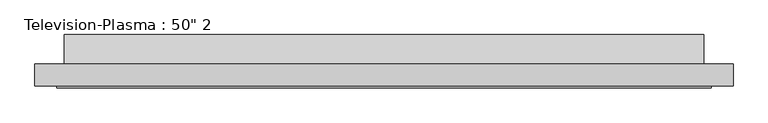
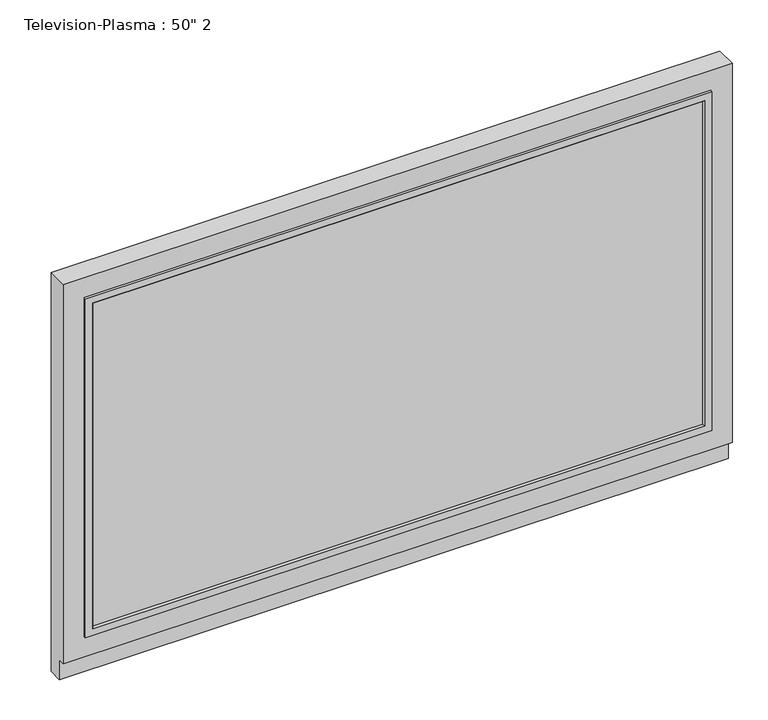
"""IFC4 building model written with IfcOpenShell, lengths in millimetres: furniture geometry."""

from ifc_helpers import new_model, si_unit, frame, origin, place, context, project, spatial, polyline, outline, extrude, faceted_brep, source, transform, mapped, element, save


def furniture_5e39d705(model_context):
    return source(origin(), model_context, "Body", "SolidModel", [
        extrude(outline(polyline([(609.6, -88.9), (-495.3, -88.9), (-495.3, -74.1720413), (609.6, -74.1720413), (609.6, -88.9)])), frame((0.0, 0.0, 88.9), z_axis=(0.0, 0.0, 1.0), x_axis=(1.0, 0.0, 0.0)), (0.0, 0.0, 1.0), 622.3),
        faceted_brep([(660.4, -50.8, 762.0), (-546.1, -50.8, 762.0), (-546.1, -88.9, 762.0), (660.4, -88.9, 762.0), (-546.1, -50.8, 0.0), (660.4, -50.8, 0.0), (660.4, -76.2, 0.0), (-546.1, -76.2, 0.0), (-495.3, -50.8, 711.2), (-495.3, -50.8, 38.1), (609.6, -50.8, 38.1), (609.6, -50.8, 711.2), (-546.1, -76.2, 38.1), (-546.1, -88.9, 38.1), (660.4, -88.9, 38.1), (-508.0, -88.9, 723.9), (622.3, -88.9, 723.9), (622.3, -88.9, 723.10625), (622.3, -88.9, 76.2), (-508.0, -88.9, 76.2), (-508.0, -88.9, 723.10625), (660.4, -76.2, 38.1), (622.3, -74.1720413, 723.9), (-508.0, -74.1720413, 723.9), (-508.0, -74.1720413, 723.10625), (622.3, -74.1720413, 723.10625), (609.6, -74.1720413, 88.9), (609.6, -74.1720413, 710.40625), (-495.3, -74.1720413, 710.40625), (-495.3, -74.1720413, 88.9), (-495.3, 0.0, 676.4688953), (-495.3, 0.0, 38.1), (609.6, 0.0, 676.4688953), (609.6, 0.0, 38.1), (606.425, -88.9, 92.075), (609.6, -92.075, 88.9), (609.6, -92.075, 710.40625), (606.425, -88.9, 707.23125), (609.6, -88.9, 88.9), (609.6, -88.9, 710.40625), (622.3, -92.075, 723.10625), (622.3, -92.075, 76.2), (-495.3, -92.075, 710.40625), (-492.125, -88.9, 707.23125), (-495.3, -88.9, 710.40625), (-508.0, -92.075, 723.10625), (-495.3, -92.075, 88.9), (-492.125, -88.9, 92.075), (-495.3, -88.9, 88.9), (-508.0, -92.075, 76.2)], [[[0, 1, 2, 3]], [[4, 5, 6, 7]], [[1, 0, 5, 4], [8, 9, 10, 11]], [[2, 1, 4, 7, 12, 13]], [[3, 2, 13, 14], [15, 16, 17, 18, 19, 20]], [[0, 3, 14, 21, 6, 5]], [[22, 23, 24, 25]], [[26, 27, 28, 29]], [[16, 22, 25, 17]], [[23, 15, 20, 24]], [[23, 22, 16, 15]], [[21, 12, 7, 6]], [[12, 21, 14, 13]], [[30, 31, 9, 8]], [[32, 11, 10, 33]], [[31, 30, 32, 33]], [[9, 31, 33, 10]], [[30, 8, 11, 32]], [[34, 35, 36, 37]], [[26, 38, 39, 27]], [[40, 41, 18, 17]], [[37, 36, 42, 43]], [[27, 39, 44, 28]], [[45, 40, 17, 25, 24, 20]], [[43, 42, 46, 47]], [[28, 44, 48, 29]], [[49, 45, 20, 19]], [[41, 40, 45, 49], [36, 35, 46, 42]], [[35, 34, 47, 46]], [[39, 38, 48, 44], [34, 37, 43, 47]], [[38, 26, 29, 48]], [[41, 49, 19, 18]]]),
    ])


if __name__ == "__main__":
    model = new_model("IFC4")
    model_context = context("Model", 3, world=origin())
    ifc_project = project(units=[si_unit("LENGTHUNIT", "METRE", prefix="MILLI")], contexts=[model_context])
    site = spatial("IfcSite", under=ifc_project)
    building = spatial("IfcBuilding", under=site)
    placement = place(None, origin())
    furniture_shape = furniture_5e39d705(model_context)
    element("IfcFurniture", 1, ObjectType="Television-Plasma : 50\" 2", at=placement, inside=building, context=model_context, shape_type="MappedRepresentation", body=[
        mapped(furniture_shape, transform((0.0, 0.0, 0.0), x_axis=(1.0, 0.0, 0.0), y_axis=(0.0, 1.0, 0.0), z_axis=(0.0, 0.0, 1.0))),
    ])
    save(model, "model.ifc")

# Revit data of these elements
# Type "Television-Plasma : 50\" 2"
#   Assembly Code = "E2020200"
#   Depth = 0' - 3 1/2"
#   Height = 2' - 6"
#   Width = 3' - 11 1/2"
#   Cabinet Material = Plastic - Gray
#   Default Elevation = 0
# Element 1 (IfcFurniture, "Television-Plasma : 50\" 2")
#   Materials on its faces: "Plastic - Gray", "Glass"
# Materials
#   "Plastic - Gray": colour RGB 134 134 134, transparency 0
#   "Glass": class "Glass", colour RGB 0 128 192, transparency 0.75, Description = "Soda Lime Glass", Cost = 0
